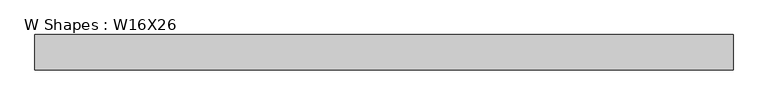
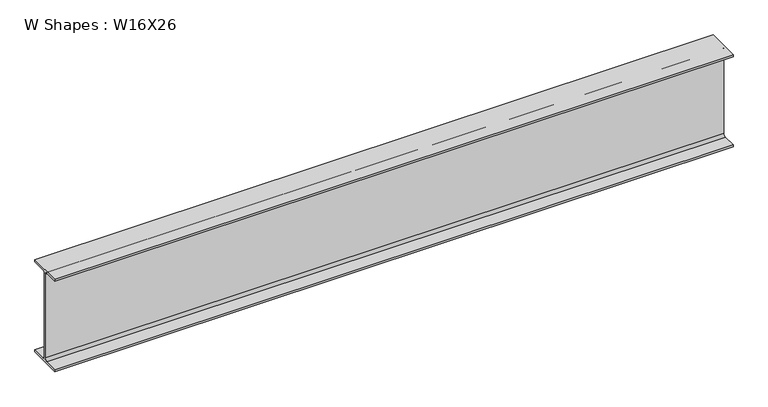
"""IFC4 building model written with IfcOpenShell, lengths in millimetres: beam geometry, W Shapes : W16X26."""

from ifc_helpers import new_model, si_unit, point, frame, frame_2d, origin, place, context, project, spatial, polyline, circle_curve, trimmed, segment, composite_curve, outline, extrude, source, transform, mapped, element, save


def w_shapes_w16x26_71b85d0e(model_context):
    return source(origin(), model_context, "Body", "SweptSolid", [
        extrude(outline(composite_curve([segment(polyline([(69.85, -190.627), (69.85, -199.39), (-69.85, -199.39), (-69.85, -190.627), (-13.3858, -190.627)]), True, "CONTINUOUS"), segment(trimmed(circle_curve(frame_2d((-13.3858, -180.4162)), 10.2108), [point((-13.3858, -190.627))], [point((-3.175, -180.4162))], True, "CARTESIAN"), True, "CONTINUOUS"), segment(polyline([(-3.175, -180.4162), (-3.175, 180.4162)]), True, "CONTINUOUS"), segment(trimmed(circle_curve(frame_2d((-13.3858, 180.4162)), 10.2108), [point((-3.175, 180.4162))], [point((-13.3858, 190.627))], True, "CARTESIAN"), True, "CONTINUOUS"), segment(polyline([(-13.3858, 190.627), (-69.85, 190.627), (-69.85, 199.39), (69.85, 199.39), (69.85, 190.627), (13.3858, 190.627)]), True, "CONTINUOUS"), segment(trimmed(circle_curve(frame_2d((13.3858, 180.4162)), 10.2108), [point((13.3858, 190.627))], [point((3.175, 180.4162))], True, "CARTESIAN"), True, "CONTINUOUS"), segment(polyline([(3.175, 180.4162), (3.175, -180.4162)]), True, "CONTINUOUS"), segment(trimmed(circle_curve(frame_2d((13.3858, -180.4162)), 10.2108), [point((3.175, -180.4162))], [point((13.3858, -190.627))], True, "CARTESIAN"), True, "CONTINUOUS"), segment(polyline([(13.3858, -190.627), (69.85, -190.627)]), True, "CONTINUOUS")], self_intersect=False)), frame((-1384.3, 0.0, 0.0), z_axis=(1.0, 0.0, 0.0), x_axis=(0.0, 1.0, 0.0)), (0.0, 0.0, 1.0), 2768.6),
    ])


if __name__ == "__main__":
    model = new_model("IFC4")
    model_context = context("Model", 3, world=origin())
    ifc_project = project(units=[si_unit("LENGTHUNIT", "METRE", prefix="MILLI")], contexts=[model_context])
    site = spatial("IfcSite", under=ifc_project)
    building = spatial("IfcBuilding", under=site)
    placement = place(None, origin())
    w_shapes_w16x26_shape = w_shapes_w16x26_71b85d0e(model_context)
    element("IfcBeam", 1, ObjectType="W Shapes : W16X26", at=placement, inside=building, context=model_context, shape_type="MappedRepresentation", body=[
        mapped(w_shapes_w16x26_shape, transform((0.0, 0.0, 0.0), x_axis=(1.0, 0.0, 0.0), y_axis=(0.0, 1.0, 0.0), z_axis=(0.0, 0.0, 1.0))),
    ])
    save(model, "model.ifc")

# Revit data of these elements
# Type "W Shapes : W16X26"
#   Section Name Key = "W16x26"
#   Assembly Code = "B10"
#   Width = 5.500"
#   Web Thickness = 0.250"
#   Web Fillet = 0.402"
#   Warping Constant = 565.00 in⁶
#   Torsional Moment of Inertia = 0.262 in⁴
#   Section Area = 7.68 in²
#   Plastic Modulus weak axis = 5.48 in³
#   Plastic Modulus strong axis = 44.20 in³
#   Perimeter = 52.20 ft²/ft
#   Nominal Weight = 26.00 lbf/ft
#   Moment of Inertia weak axis = 9.59 in⁴
#   Moment of Inertia strong axis = 301.00 in⁴
#   Height = 15.700"
#   Flange Thickness = 0.345"
#   Elastic Modulus weak axis = 3.49 in³
#   Elastic Modulus strong axis = 38.40 in³
#   Centroid Vertical = 7.850"
#   Centroid Horizontal = 2.750"
#   Bolt Spacing = 0' - 3 1/2"
#   Length [instance default] = 5' - 0"
#   Structural Material [instance default] = Steel ASTM A992
#   Principal Axes Angle = 0
# Element 1 (IfcBeam, "W Shapes : W16X26")
#   Materials on its faces: "Steel ASTM A992"
# Materials
#   "Steel ASTM A992": class "Metal", colour RGB 199 199 199, transparency 0, Description = "Structural steel 50ksi", Cost = 0
